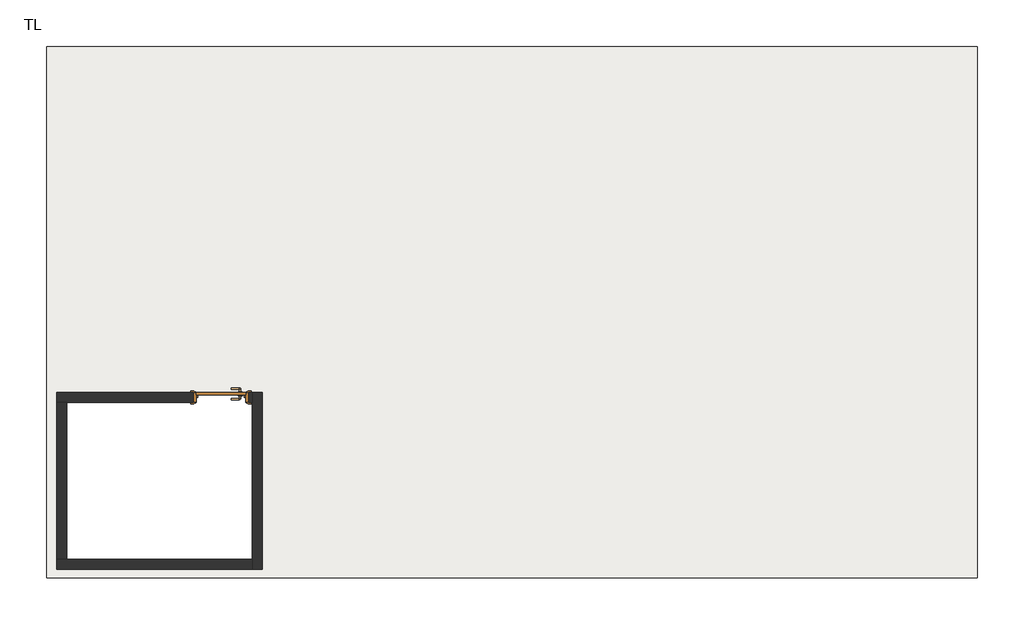
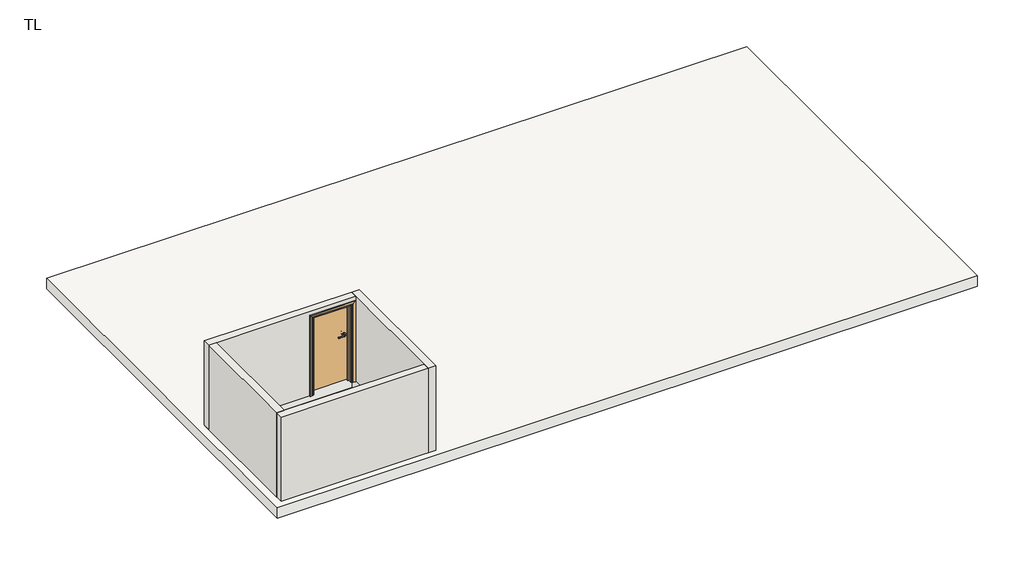
# One storey, incomplete: 4 walls, 1 door, 1 slab.
"""IFC4 building model written with IfcOpenShell, lengths in millimetres."""

from ifc_helpers import new_model, si_unit, frame, origin, place, context, project, spatial, polyline, outline, extrude, faceted_brep, transform, mapped, element, save
from components import doors_intsgl_out_door1_d16f2837

model = new_model("IFC4")

# Units and contexts
model_context = context("Model", 3, world=origin())
ifc_project = project(units=[si_unit("LENGTHUNIT", "METRE", prefix="MILLI")], contexts=[model_context])

# Site, building, storey
site = spatial("IfcSite", under=ifc_project)
building = spatial("IfcBuilding", under=site)
storey = spatial("IfcBuildingStorey", under=building, Name="TL", Elevation=3048.0)

# Door
placement = place(None, origin())
doors_intsgl_out_door1_shape = doors_intsgl_out_door1_d16f2837(model_context)
element("IfcDoor", 1, ObjectType="Doors_IntSgl : OUT DOOR1", at=placement, inside=storey, context=model_context, shape_type="MappedRepresentation", body=[
    mapped(doors_intsgl_out_door1_shape, transform((-2149.4596772, 1993.3922428, 3247.9488), x_axis=(-1.0, 0.0, 0.0), y_axis=(0.0, -1.0, 0.0), z_axis=(0.0, 0.0, 1.0))),
])

# Slab
element("IfcSlab", 2, ObjectType="SLAB FLOOR", at=placement, inside=storey, context=model_context, shape_type="SweptSolid", body=[
    extrude(outline(polyline([(8253.9722582, 6821.9322428), (8253.9722582, -493.2677572), (-4547.6277418, -493.2677572), (-4547.6277418, 6821.9322428), (8253.9722582, 6821.9322428)]), holes=[polyline([(-4410.4677418, -234.1877572), (-1717.6596772, -234.1877572), (-1717.6596772, 2042.8185606), (-4410.4677418, 2042.8185606), (-4410.4677418, -234.1877572)])]), frame((0.0, 0.0, 3048.0), z_axis=(0.0, 0.0, 1.0), x_axis=(1.0, 0.0, 0.0)), (0.0, 0.0, 1.0), 199.9488),
])

# Walls
element("IfcWall", 3, ObjectType="INNER WALL", at=placement, inside=storey, context=model_context, shape_type="Brep", body=[
    faceted_brep([(-1580.4996772, -371.3477572, 3247.9488), (-1580.4996772, 2061.9722428, 3247.9488), (-1580.4996772, 2061.9722428, 4876.8), (-1580.4996772, -371.3477572, 4876.8), (-1717.6596772, -371.3477572, 3247.9488), (-1717.6596772, -371.3477572, 4876.8), (-1717.6596772, -234.1877572, 4876.8), (-1717.6596772, 1924.8122428, 4876.8), (-1717.6596772, 2061.9722428, 4876.8), (-1717.6596772, 2061.9722428, 3247.9488), (-1717.6596772, 1924.8122428, 3247.9488), (-1717.6596772, -234.1877572, 3247.9488)], [[[0, 1, 2, 3]], [[4, 5, 6, 7, 8, 9, 10, 11]], [[1, 0, 4, 11, 10, 9]], [[3, 2, 8, 7, 6, 5]], [[0, 3, 5, 4]], [[2, 1, 9, 8]]]),
])
element("IfcWall", 4, ObjectType="INNER WALL", at=placement, inside=storey, context=model_context, shape_type="Brep", body=[
    faceted_brep([(-1717.6596772, -234.1877572, 3247.9488), (-4270.7677418, -234.1877572, 3247.9488), (-4407.9277418, -234.1877572, 3247.9488), (-4407.9277418, -234.1877572, 4876.8), (-4270.7677418, -234.1877572, 4876.8), (-1717.6596772, -234.1877572, 4876.8), (-1717.6596772, -371.3477572, 3247.9488), (-1717.6596772, -371.3477572, 4876.8), (-4407.9277418, -371.3477572, 4876.8), (-4407.9277418, -371.3477572, 3247.9488)], [[[0, 1, 2, 3, 4, 5]], [[6, 7, 8, 9]], [[2, 1, 0, 6, 9]], [[5, 4, 3, 8, 7]], [[0, 5, 7, 6]], [[3, 2, 9, 8]]]),
])
element("IfcWall", 5, ObjectType="INNER WALL", at=placement, inside=storey, context=model_context, shape_type="SweptSolid", body=[
    extrude(outline(polyline([(-4407.9277418, -234.1877572), (-4407.9277418, 1920.8985606), (-4270.7677418, 1920.8985606), (-4270.7677418, -234.1877572), (-4407.9277418, -234.1877572)])), frame((0.0, 0.0, 3247.9488), z_axis=(0.0, 0.0, 1.0), x_axis=(1.0, 0.0, 0.0)), (0.0, 0.0, 1.0), 1628.8512),
])
element("IfcWall", 6, ObjectType="INNER WALL", at=placement, inside=storey, context=model_context, shape_type="SweptSolid", body=[
    extrude(outline(polyline([(4876.8, -4410.4677418), (3247.9488, -4410.4677418), (3247.9488, -2530.4596772), (4771.9488, -2530.4596772), (4771.9488, -1768.4596772), (3247.9488, -1768.4596772), (3247.9488, -1717.6596772), (4876.8, -1717.6596772), (4876.8, -4410.4677418)])), frame((0.0, 1924.8122428, 0.0), z_axis=(0.0, 1.0, 0.0), x_axis=(0.0, 0.0, 1.0)), (0.0, 0.0, 1.0), 137.16),
])

save(model, "model.ifc")

# Revit data of these elements
# Type "Doors_IntSgl : OUT DOOR1"
#   Type Mark = "53"
#   Type Comments = "Internal Single"
#   Operation = "SingleSwingRight"
#   Manufacturer = "Revit"
#   Keynote = "L20"
#   Description = "Internal Single Door"
#   Analytic Construction = "Metal"
#   UnderCut = 8 mm
#   Tolerance = 2 mm
#   Thickness = 38 mm
#   Thermal Resistance (R) = 0.270117 (m²·K)/W
#   Structural Tolerance = 8 mm
#   StopDepth = 32 mm
#   Stop Thickness = 19 mm
#   Rough Width = 762 mm
#   Rough Height = 1524 mm
#   Height to Top Lock Rail = 1000 mm
#   Heat Transfer Coefficient (U) = 3.7021 W/(m²·K)
#   Handle Z Distance = 900 mm
#   Handle X Distance = 75 mm
#   Frame Thickness = 32 mm
#   Door Panel Width = 678 mm
#   Door Panel Thickness = 38 mm
#   Door Panel Offset = 0 mm
#   Height = 1524 mm
#   Width = 762 mm
#   Door Panel Height = 1474 mm
#   Architrave Setback = 5 mm
#   Vis - Ironmongery = yes
#   Material Ironmongery = Door - Handle
#   Material Frame = Door - Frame/Mullion (1)
#   Material Door = Door - Panel
#   Material Architrave = Door - Architrave
#   Visual Light Transmittance = 0
#   Solar Heat Gain Coefficient = 0
#   Function = (empty or 0)
#   Wall Closure = (empty or 0)
# Type "SLAB FLOOR"
#   Layers, outside or top first: 199.949 mm "Concrete, Precast" (function 1)
# Type "INNER WALL"
#   Keynote = "F10"
#   Layers, outside or top first: 137.16 mm "Brick, Common" (function 1)
# Element 1 (IfcDoor, "Doors_IntSgl : OUT DOOR1")
#   Phase Created = New Construction
#   Materials on its faces: "Door - Architrave", "Door - Handle", "Door - Frame/Mullion (1)", "Door - Panel"
# Element 2 (IfcSlab, "SLAB FLOOR")
#   Height Offset From Level = 199.949 mm
#   built-in parameter 1001954 = 1
#   Phase Created = New Construction
#   Materials on its faces: "Concrete, Precast"
# Elements 3, 4, 5, 6 (IfcWall, "INNER WALL")
#   built-in parameter 1001111 = 199.949 mm
#   Top Offset = 0 mm
#   Base Offset = 199.949 mm
#   Unconnected Height = 1628.851 mm
#   wall height = 1628.851 mm
#   Phase Created = New Construction
#   Base Constraint = TL
#   Materials on its faces: "Brick, Common"
# Materials
#   "Door - Handle": colour RGB 0 0 0, transparency 0, Keynote = "P21", Cost = 0
#   "Door - Frame/Mullion (1)": class "Wood", colour RGB 212 179 113, transparency 0, Keynote = "L20", Cost = 0
#   "Door - Panel": class "Wood", colour RGB 210 159 95, transparency 0, Keynote = "L20", Cost = 0
#   "Door - Architrave": class "Wood", colour RGB 154 90 5, transparency 0, Keynote = "P20", Cost = 0
#   "Concrete, Precast": class "Concrete", colour RGB 192 192 192, transparency 0, Description = "Precast concrete", Cost = 0
#   "Brick, Common": class "Masonry", colour RGB 170 100 105, transparency 0, Description = "Common brick", Cost = 0
